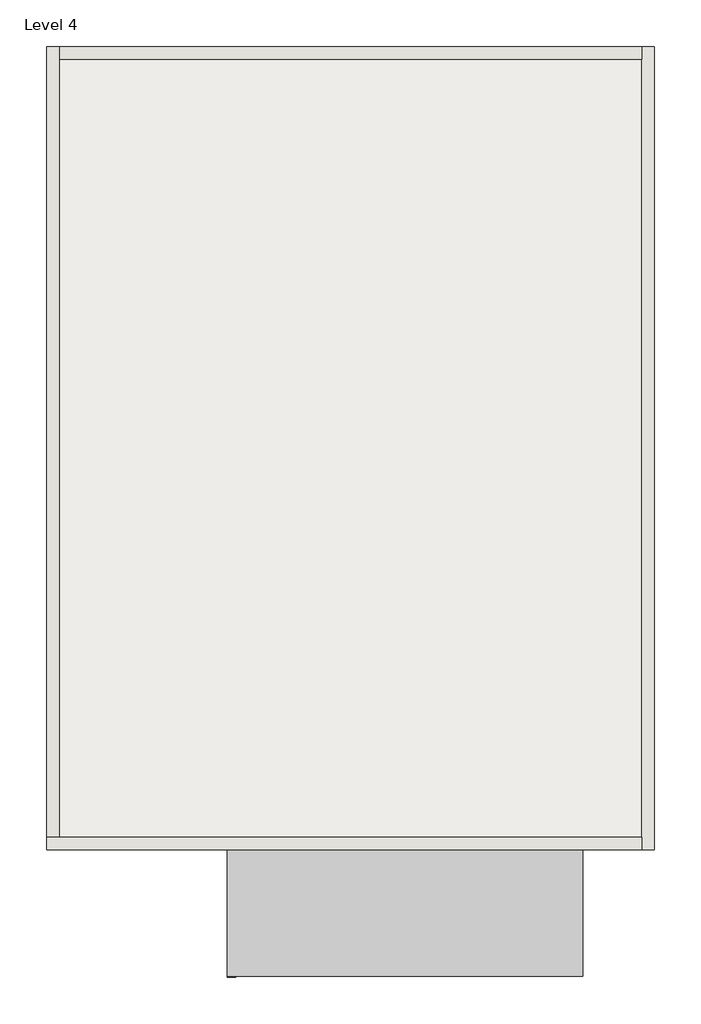
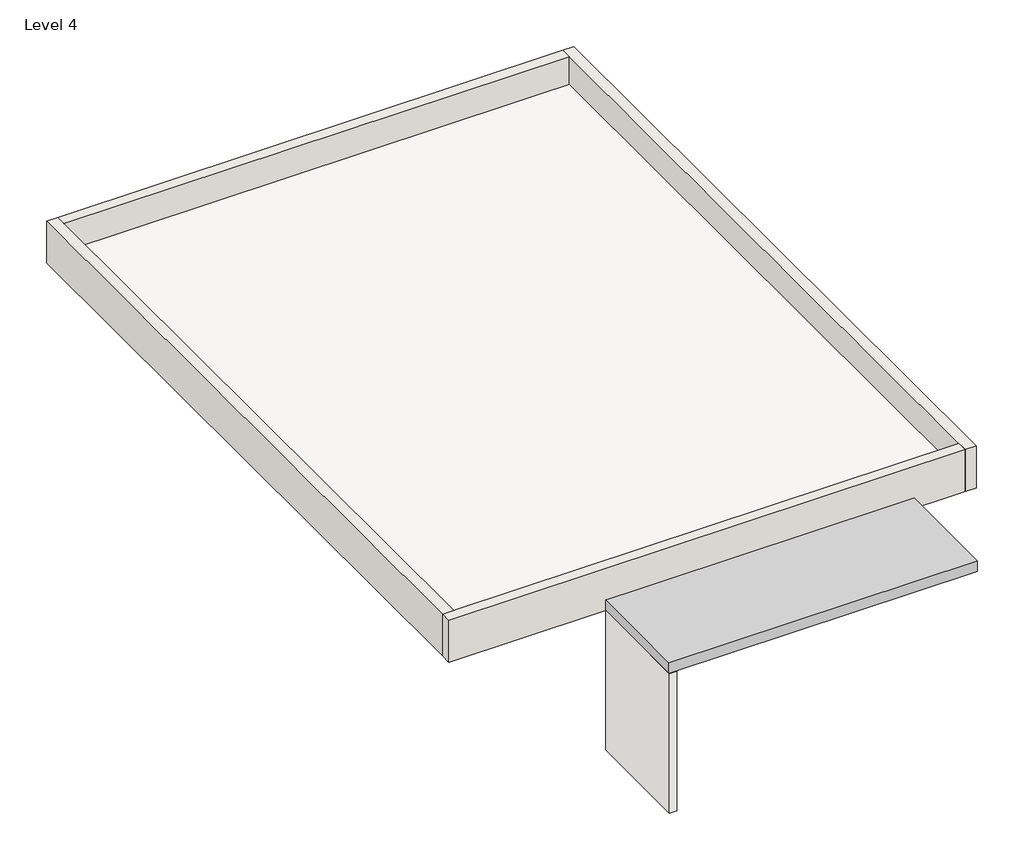
# One storey: 4 walls, 1 proxy, 1 roof, 1 slab.
"""IFC4 building model written with IfcOpenShell, lengths in millimetres."""

from ifc_helpers import new_model, si_unit, frame, origin, place, context, project, spatial, polyline, outline, extrude, faceted_brep, transform, mapped, element, save
from components import generic_models_5_generic_models_5_d5554940, floors_1_floors_1_82467aff

model = new_model("IFC4")

# Units and contexts
model_context = context("Model", 3, world=origin())
ifc_project = project(units=[si_unit("LENGTHUNIT", "METRE", prefix="MILLI")], contexts=[model_context])

# Site, building, storey
site = spatial("IfcSite", under=ifc_project)
building = spatial("IfcBuilding", under=site)
storey = spatial("IfcBuildingStorey", under=building, Name="Level 4", Elevation=6400.8)

# Proxy
placement = place(None, origin())
generic_models_5_generic_models_5_shape = generic_models_5_generic_models_5_d5554940(model_context)
element("IfcBuildingElementProxy", 1, Name="Generic Models 5 : Generic Models 5", ObjectType="Generic Models 5 : Generic Models 5", at=placement, inside=storey, context=model_context, shape_type="MappedRepresentation", body=[
    mapped(generic_models_5_generic_models_5_shape, transform((0.0, 0.0, 0.0), x_axis=(1.0, 0.0, 0.0), y_axis=(0.0, 1.0, 0.0), z_axis=(0.0, 0.0, 1.0))),
])

# Roof
element("IfcRoof", 2, ObjectType="ROOFING 6\"", at=placement, inside=storey, context=model_context, shape_type="SweptSolid", body=[
    extrude(outline(polyline([(-6528.0474631, 9900.9061648), (3912.9151699, 9900.9061648), (3912.9151699, -4043.6938352), (-6528.0474631, -4043.6938352), (-6528.0474631, 9900.9061648)])), frame((0.0, 0.0, 6400.8), z_axis=(0.0, 0.0, 1.0), x_axis=(1.0, 0.0, 0.0)), (0.0, 0.0, 1.0), 304.8),
])

# Slab
floors_1_floors_1_shape = floors_1_floors_1_82467aff(model_context)
element("IfcSlab", 3, ObjectType="Floors 1 : Floors 1", at=placement, inside=storey, context=model_context, shape_type="MappedRepresentation", body=[
    mapped(floors_1_floors_1_shape, transform((0.0, 0.0, 0.0), x_axis=(1.0, 0.0, 0.0), y_axis=(0.0, 1.0, 0.0), z_axis=(0.0, 0.0, 1.0))),
])

# Walls
element("IfcWall", 4, ObjectType="EXTERIOR WALL 9\"", at=placement, inside=storey, context=model_context, shape_type="Brep", body=[
    faceted_brep([(3911.3525369, 10129.5061648, 6400.8), (3911.3525369, 9900.9061648, 6400.8), (3911.3525369, -4043.6938352, 6400.8), (3911.3525369, -4272.2938352, 6400.8), (3911.3525369, -4272.2938352, 7315.2), (3911.3525369, -4043.6938352, 7315.2), (3911.3525369, 9900.9061648, 7315.2), (3911.3525369, 10129.5061648, 7315.2), (4139.9525369, 10129.5061648, 6400.8), (4139.9525369, 10129.5061648, 7315.2), (4139.9525369, -4272.2938352, 7315.2), (4139.9525369, -4272.2938352, 6400.8)], [[[0, 1, 2, 3, 4, 5, 6, 7]], [[8, 9, 10, 11]], [[3, 2, 1, 0, 8, 11]], [[7, 6, 5, 4, 10, 9]], [[4, 3, 11, 10]], [[0, 7, 9, 8]]]),
])
element("IfcWall", 5, ObjectType="EXTERIOR WALL 9\"", at=placement, inside=storey, context=model_context, shape_type="Brep", body=[
    faceted_brep([(3911.3525369, -4043.6938352, 6400.8), (-6528.0474631, -4043.6938352, 6400.8), (-6756.6474631, -4043.6938352, 6400.8), (-6756.6474631, -4043.6938352, 7315.2), (-6528.0474631, -4043.6938352, 7315.2), (3911.3525369, -4043.6938352, 7315.2), (3911.3525369, -4272.2938352, 6400.8), (3911.3525369, -4272.2938352, 7315.2), (-6756.6474631, -4272.2938352, 7315.2), (-6756.6474631, -4272.2938352, 6400.8)], [[[0, 1, 2, 3, 4, 5]], [[6, 7, 8, 9]], [[2, 1, 0, 6, 9]], [[5, 4, 3, 8, 7]], [[0, 5, 7, 6]], [[3, 2, 9, 8]]]),
])
element("IfcWall", 6, ObjectType="EXTERIOR WALL 9\"", at=placement, inside=storey, context=model_context, shape_type="Brep", body=[
    faceted_brep([(-6528.0474631, -4043.6938352, 6400.8), (-6528.0474631, 9900.9061648, 6400.8), (-6528.0474631, 10129.5061648, 6400.8), (-6528.0474631, 10129.5061648, 7315.2), (-6528.0474631, 9900.9061648, 7315.2), (-6528.0474631, -4043.6938352, 7315.2), (-6756.6474631, -4043.6938352, 6400.8), (-6756.6474631, -4043.6938352, 7315.2), (-6756.6474631, 10129.5061648, 7315.2), (-6756.6474631, 10129.5061648, 6400.8)], [[[0, 1, 2, 3, 4, 5]], [[6, 7, 8, 9]], [[2, 1, 0, 6, 9]], [[5, 4, 3, 8, 7]], [[0, 5, 7, 6]], [[3, 2, 9, 8]]]),
])
element("IfcWall", 7, ObjectType="EXTERIOR WALL 9\"", at=placement, inside=storey, context=model_context, shape_type="SweptSolid", body=[
    extrude(outline(polyline([(3911.3525369, 9900.9061648), (-6528.0474631, 9900.9061648), (-6528.0474631, 10129.5061648), (3911.3525369, 10129.5061648), (3911.3525369, 9900.9061648)])), frame((0.0, 0.0, 6400.8), z_axis=(0.0, 0.0, 1.0), x_axis=(1.0, 0.0, 0.0)), (0.0, 0.0, 1.0), 914.4),
])

save(model, "model.ifc")

# Revit data of these elements
# Type "ROOFING 6\""
#   Assembly Code = "B1020"
#   Layers, outside or top first: 1' - 0" "ROOFING" (function 1)
# Type "EXTERIOR WALL 9\""
#   Assembly Code = "B2010"
#   Layers, outside or top first: 0' - 9" "OFF WHITE COLOUR" (function 1)
# Element 1 (IfcBuildingElementProxy, "Generic Models 5 : Generic Models 5")
#   Phase Created = New Construction
#   Materials on its faces: "WALL PAINT"
# Element 2 (IfcRoof, "ROOFING 6\"")
#   built-in parameter 1001705 = 22 (stored number, unit not read)
#   built-in parameter 1001710 = 33615
#   Phase Created = New Construction
#   Materials on its faces: "ROOFING"
# Element 3 (IfcSlab, "Floors 1 : Floors 1")
#   Phase Created = New Construction
#   Materials on its faces: "WALL PAINT"
# Elements 4, 5, 6, 7 (IfcWall, "EXTERIOR WALL 9\"")
#   Top Offset = 0' - 0"
#   Base Offset = 0' - 0"
#   Unconnected Height = 3' - 0"
#   wall height = 3' - 0"
#   Phase Created = New Construction
#   Base Constraint = Level 4
#   Materials on its faces: "OFF WHITE COLOUR"
# Materials
#   "ROOFING": class "Generic", colour RGB 120 120 120, transparency 0, Cost = 0
#   "OFF WHITE COLOUR": class "Generic", colour RGB 120 120 120, transparency 0, Cost = 0
#   "WALL PAINT": class "Generic", colour RGB 120 120 120, transparency 0, Cost = 0
